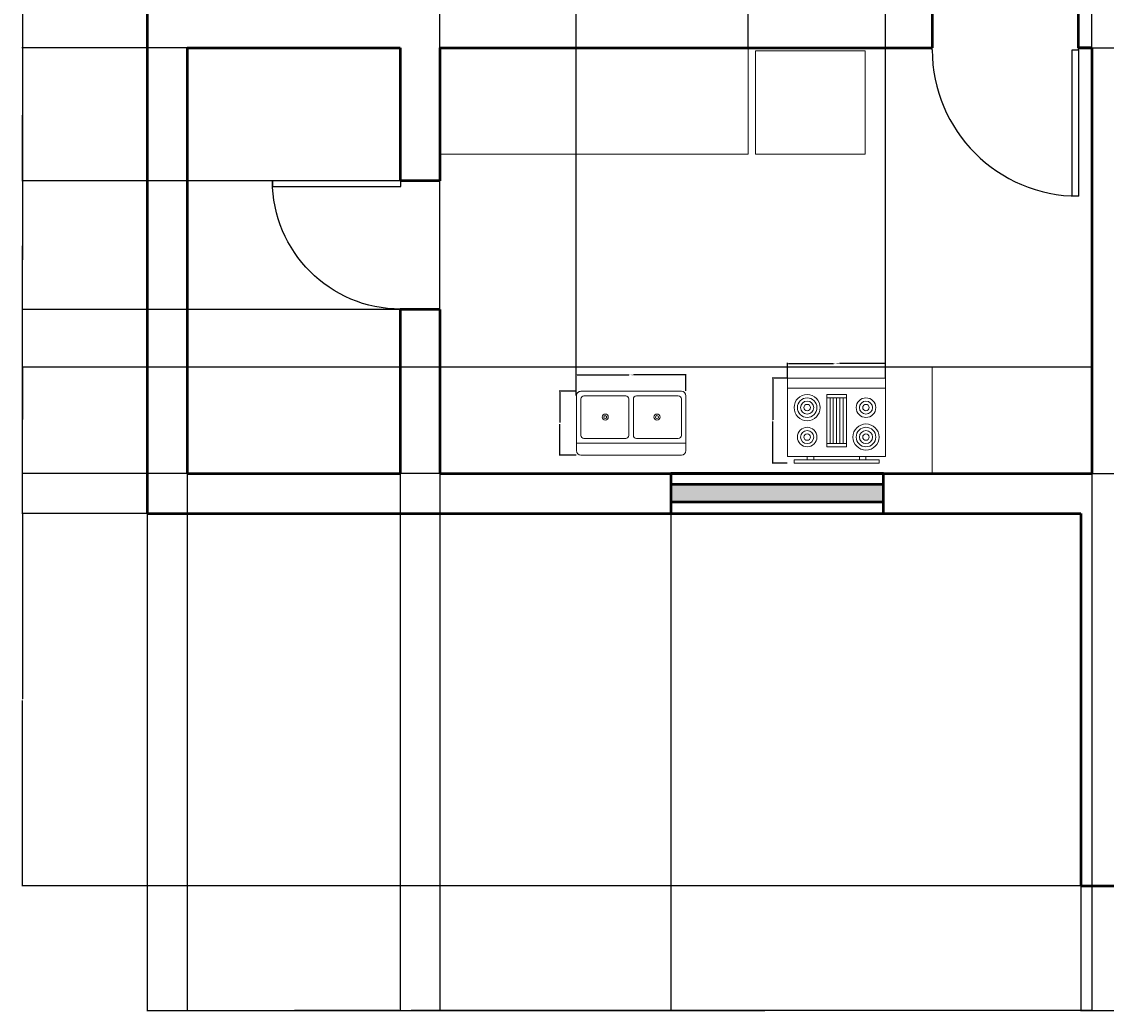
# Model space of a CAD drawing. Units: inches. Extents: x 1974 to 2406, y 1583 to 2170.
# Tile 1 of 6: x 1974 to 2218, y 1583 to 1806. Entities that reach past the tile are written whole.
import ezdxf

# ---------------------------------------------------------------- set-up
doc = ezdxf.new("R2010")
doc.units = ezdxf.units.IN
for name, color, linetype, lineweight in [('A-ANNO-DIMS', 2, 'Continuous', 18), ('A-EQPM', 3, 'Continuous', 18), ('A-FLOR-FIXT', 3, 'Continuous', 18), ('A-GLAZ', 4, 'Continuous', 25), ('door', 60, 'Continuous', 25), ('wall', 240, 'Continuous', 50)]:
    doc.layers.add(name, color=color, linetype=linetype, lineweight=lineweight)
doc.layers.add('A-FLOR-CASE', color=40, linetype='Continuous', lineweight=18, true_color=0xf8d731)
doc.styles.get("Standard").update_dxf_attribs({"font": 'arial.ttf'})
doc.dimstyles.get("Standard").update_dxf_attribs({"dimtxt": 0.18, "dimasz": 0.18, "dimexe": 0.18, "dimexo": 0.0625, "dimgap": 0.09, "dimtad": 0, "dimtih": 1, "dimtoh": 1, "dimdec": 4, "dimzin": 0, "dimdsep": 46, "dimtxsty": 'Standard', "dimcen": 0.09, "dimadec": 0, "dimazin": 0, "dimtfac": 1, "dimtdec": 4, "dimtofl": 0, "dimtmove": 0, "dimatfit": 3, "dimfxl": 1, "dimtolj": 1, "dimtzin": 0, "dimarcsym": 0})

# ---------------------------------------------------------------- blocks, each defined once
blk = doc.blocks.new('*U2')
for p, q in [((0, 0), (0, -6)), ((40, 0), (40, -6))]:
    blk.add_line(p, q)
blk.add_lwpolyline([(0, 0), (0, 40), (1.75, 40), (1.75, 0)], close=True)
blk.add_arc((0, 0), 40, 0, 90)
blk = doc.blocks.new('b')
at = {"layer": 'wall'}
h = blk.add_hatch(color=256, dxfattribs=at)
h.dxf.hatch_style = 1
h.paths.add_polyline_path([(6.5, 0), (2.5, 0), (2.5, -48), (6.5, -48)])
for p, q in [((2.5, 0), (2.5, -48)), ((6.5, 0), (6.5, -48))]:
    blk.add_line(p, q, dxfattribs=at)
blk.add_lwpolyline([(0, -48), (9, -48), (9, 0), (0, 0)], close=True, dxfattribs=at)
blk = doc.blocks.new('Sink-double - 36 in top')
for p, q in [((-18, -4), (18, -4)), ((-0.75, -18.5), (-0.75, -6.5)), ((0.75, -6.5), (0.75, -18.5))]:
    blk.add_line(p, q)
for points in [[(-16.5, 0), (16.5, 0)], [(-18, -19.5), (-18, -1.5)], [(18, -1.5), (18, -19.5)], [(-16.5, -18.5), (-16.5, -6.5)], [(-15.5, -5.5), (-1.75, -5.5)], [(1.75, -5.5), (15.5, -5.5)], [(16.5, -6.5), (16.5, -18.5)], [(16.5, -21), (-16.5, -21)], [(-1.75, -19.5), (-15.5, -19.5)], [(15.5, -19.5), (1.75, -19.5)]]:
    blk.add_lwpolyline(points)
for centre, radius in [((-8.5, -12.5), 1), ((-8.5, -12.5), 0.5), ((8.5, -12.5), 1), ((8.5, -12.5), 0.5)]:
    blk.add_circle(centre, radius)
for centre, radius, start, end in [((-16.5, -1.5), 1.5, 90, 180), ((16.5, -1.5), 1.5, 0, 90), ((-15.5, -6.5), 1, 90, 180), ((-1.75, -6.5), 1, 0, 90), ((1.75, -6.5), 1, 90, 180), ((15.5, -6.5), 1, 0, 90), ((-16.5, -19.5), 1.5, 180, 270), ((-15.5, -18.5), 1, 180, 270), ((-1.75, -18.5), 1, 270, 0), ((1.75, -18.5), 1, 180, 270), ((15.5, -18.5), 1, 270, 0), ((16.5, -19.5), 1.5, 270, 0)]:
    blk.add_arc(centre, radius, start, end)
blk = doc.blocks.new('Range-Oven - 30 in top')
for p, q in [((0, -3), (30, -3)), ((12, -6), (18, -6)), ((13, -20), (13, -6)), ((14, -6), (14, -20)), ((15, -20), (15, -6)), ((16, -6), (16, -20)), ((17, -20), (17, -6)), ((18, -20), (12, -20)), ((6, -24), (6, -25)), ((8, -25), (8, -24)), ((22, -25), (22, -24)), ((24, -24), (24, -25))]:
    blk.add_line(p, q)
for points in [[(0, -24), (0, 0), (30, 0), (30, -24)], [(12, -21), (12, -5), (18, -5), (18, -21)], [(2, -26), (2, -25), (28, -25), (28, -26)]]:
    blk.add_lwpolyline(points, close=True)
for centre, radius in [((6, -9), 4), ((6, -9), 3), ((24, -9), 3), ((6, -9), 2), ((6, -9), 1), ((24, -9), 2), ((24, -9), 1), ((6, -18), 3), ((6, -18), 2), ((24, -18), 4), ((24, -18), 3), ((24, -18), 2), ((6, -18), 1), ((24, -18), 1)]:
    blk.add_circle(centre, radius)
blk = doc.blocks.new('*D38')
at = {"layer": 'A-ANNO-DIMS', "color": 0, "lineweight": -2, "transparency": 16777216}
for p, q in [((2098.9, 1722.59), (2098.9, 1726.41)), ((2099.08, 1726.23), (2110.71, 1726.23)), ((2123.43, 1726.23), (2111.81, 1726.23)), ((2123.61, 1722.59), (2123.61, 1726.41))]:
    blk.add_line(p, q, dxfattribs=at)
at = {"layer": 'A-ANNO-DIMS', "color": 0, "transparency": 16777216}
for points in [[(2099.08, 1726.26), (2099.08, 1726.2), (2098.9, 1726.23)], [(2123.43, 1726.26), (2123.43, 1726.2), (2123.61, 1726.23)]]:
    blk.add_solid(points, dxfattribs=at)
at = {"layer": 'Defpoints', "color": 0, "transparency": 16777216}
for p in [(2098.9, 1726.23), (2098.9, 1722.52), (2123.61, 1722.52)]:
    blk.add_point(p, dxfattribs=at)
at = {"layer": 'A-ANNO-DIMS', "color": 0, "transparency": 16777216, "insert": (2111.26, 1726.23), "char_height": 0.18, "attachment_point": 5}
blk.add_mtext('\\A1;SINK 25', dxfattribs=at)
blk = doc.blocks.new('*D39')
at = {"layer": 'A-ANNO-DIMS', "color": 0, "lineweight": -2, "transparency": 16777216}
for p, q in [((2098.84, 1722.52), (2095.02, 1722.52)), ((2095.2, 1722.34), (2095.2, 1715.5)), ((2095.2, 1708.29), (2095.2, 1715.14)), ((2098.84, 1708.11), (2095.02, 1708.11))]:
    blk.add_line(p, q, dxfattribs=at)
at = {"layer": 'A-ANNO-DIMS', "color": 0, "transparency": 16777216}
for points in [[(2095.17, 1722.34), (2095.23, 1722.34), (2095.2, 1722.52)], [(2095.17, 1708.29), (2095.23, 1708.29), (2095.2, 1708.11)]]:
    blk.add_solid(points, dxfattribs=at)
at = {"layer": 'Defpoints', "color": 0, "transparency": 16777216}
for p in [(2098.9, 1722.52), (2095.2, 1708.11), (2098.9, 1708.11)]:
    blk.add_point(p, dxfattribs=at)
at = {"layer": 'A-ANNO-DIMS', "color": 0, "transparency": 16777216, "insert": (2095.2, 1715.32), "char_height": 0.18, "attachment_point": 5}
blk.add_mtext('\\A1;14', dxfattribs=at)
blk = doc.blocks.new('*D46')
at = {"layer": 'A-ANNO-DIMS', "color": 0, "lineweight": -2, "transparency": 16777216}
for p, q in [((2146.53, 1725.52), (2146.53, 1728.96)), ((2146.71, 1728.78), (2156.89, 1728.78)), ((2168.46, 1728.78), (2158.28, 1728.78)), ((2168.64, 1725.52), (2168.64, 1728.96))]:
    blk.add_line(p, q, dxfattribs=at)
at = {"layer": 'A-ANNO-DIMS', "color": 0, "transparency": 16777216}
for points in [[(2146.71, 1728.81), (2146.71, 1728.75), (2146.53, 1728.78)], [(2168.46, 1728.81), (2168.46, 1728.75), (2168.64, 1728.78)]]:
    blk.add_solid(points, dxfattribs=at)
at = {"layer": 'Defpoints', "color": 0, "transparency": 16777216}
for p in [(2168.64, 1728.78), (2146.53, 1725.46), (2168.64, 1725.46)]:
    blk.add_point(p, dxfattribs=at)
at = {"layer": 'A-ANNO-DIMS', "color": 0, "transparency": 16777216, "insert": (2157.58, 1728.78), "char_height": 0.18, "attachment_point": 5}
blk.add_mtext('\\A1;RANGE 22', dxfattribs=at)
blk = doc.blocks.new('*D47')
at = {"layer": 'A-ANNO-DIMS', "color": 0, "lineweight": -2, "transparency": 16777216}
for p, q in [((2146.47, 1725.46), (2143.03, 1725.46)), ((2143.21, 1725.28), (2143.21, 1716.06)), ((2143.21, 1706.48), (2143.21, 1715.7)), ((2146.47, 1706.3), (2143.03, 1706.3))]:
    blk.add_line(p, q, dxfattribs=at)
at = {"layer": 'A-ANNO-DIMS', "color": 0, "transparency": 16777216}
for points in [[(2143.18, 1725.28), (2143.24, 1725.28), (2143.21, 1725.46)], [(2143.18, 1706.48), (2143.24, 1706.48), (2143.21, 1706.3)]]:
    blk.add_solid(points, dxfattribs=at)
at = {"layer": 'Defpoints', "color": 0, "transparency": 16777216}
for p in [(2143.21, 1725.46), (2146.53, 1725.46), (2146.53, 1706.3)]:
    blk.add_point(p, dxfattribs=at)
at = {"layer": 'A-ANNO-DIMS', "color": 0, "transparency": 16777216, "insert": (2143.21, 1715.88), "char_height": 0.18, "attachment_point": 5}
blk.add_mtext('\\A1;19', dxfattribs=at)
blk = doc.blocks.new('*D57')
at = {"layer": 'A-ANNO-DIMS', "color": 0, "lineweight": -2, "transparency": 16777216}
for p, q in [((2011.1, 1808.99), (1973.86, 1808.99)), ((1974.04, 1808.81), (1974.04, 1752.17)), ((1974.04, 1695.17), (1974.04, 1751.81)), ((2002.1, 1694.99), (1973.86, 1694.99))]:
    blk.add_line(p, q, dxfattribs=at)
at = {"layer": 'A-ANNO-DIMS', "color": 0, "transparency": 16777216}
for points in [[(1974.01, 1808.81), (1974.07, 1808.81), (1974.04, 1808.99)], [(1974.01, 1695.17), (1974.07, 1695.17), (1974.04, 1694.99)]]:
    blk.add_solid(points, dxfattribs=at)
at = {"layer": 'Defpoints', "color": 0, "transparency": 16777216}
for p in [(2011.16, 1808.99), (1974.04, 1694.99), (2002.16, 1694.99)]:
    blk.add_point(p, dxfattribs=at)
at = {"layer": 'A-ANNO-DIMS', "color": 0, "transparency": 16777216, "insert": (1974.04, 1751.99), "char_height": 0.18, "attachment_point": 5}
blk.add_mtext('\\A1;114', dxfattribs=at)
blk = doc.blocks.new('*D58')
at = {"layer": 'A-ANNO-DIMS', "color": 0, "lineweight": -2, "transparency": 16777216}
for p, q in [((2002.1, 1694.99), (1973.86, 1694.99)), ((1974.04, 1694.81), (1974.04, 1653.17)), ((1974.04, 1611.17), (1974.04, 1652.81)), ((2212.6, 1610.99), (1973.86, 1610.99))]:
    blk.add_line(p, q, dxfattribs=at)
at = {"layer": 'A-ANNO-DIMS', "color": 0, "transparency": 16777216}
for points in [[(1974.01, 1694.81), (1974.07, 1694.81), (1974.04, 1694.99)], [(1974.01, 1611.17), (1974.07, 1611.17), (1974.04, 1610.99)]]:
    blk.add_solid(points, dxfattribs=at)
at = {"layer": 'Defpoints', "color": 0, "transparency": 16777216}
for p in [(2002.16, 1694.99), (1974.04, 1610.99), (2212.66, 1610.99)]:
    blk.add_point(p, dxfattribs=at)
at = {"layer": 'A-ANNO-DIMS', "color": 0, "transparency": 16777216, "insert": (1974.04, 1652.99), "char_height": 0.18, "attachment_point": 5}
blk.add_mtext('\\A1;84', dxfattribs=at)
blk = doc.blocks.new('*D61')
at = {"layer": 'A-ANNO-DIMS', "color": 0, "lineweight": -2, "transparency": 16777216}
for p, q in [((2002.16, 1694.93), (2002.16, 1582.69)), ((2212.66, 1610.93), (2212.66, 1582.69)), ((2002.34, 1582.87), (2107.01, 1582.87)), ((2212.48, 1582.87), (2107.8, 1582.87))]:
    blk.add_line(p, q, dxfattribs=at)
at = {"layer": 'A-ANNO-DIMS', "color": 0, "transparency": 16777216}
for points in [[(2002.34, 1582.9), (2002.34, 1582.84), (2002.16, 1582.87)], [(2212.48, 1582.9), (2212.48, 1582.84), (2212.66, 1582.87)]]:
    blk.add_solid(points, dxfattribs=at)
at = {"layer": 'Defpoints', "color": 0, "transparency": 16777216}
for p in [(2002.16, 1694.99), (2212.66, 1610.99), (2212.66, 1582.87)]:
    blk.add_point(p, dxfattribs=at)
at = {"layer": 'A-ANNO-DIMS', "color": 0, "transparency": 16777216, "insert": (2107.41, 1582.87), "char_height": 0.18, "attachment_point": 5}
blk.add_mtext('\\A1;210.5', dxfattribs=at)
blk = doc.blocks.new('*D62')
at = {"layer": 'A-ANNO-DIMS', "color": 0, "lineweight": -2, "transparency": 16777216}
for p, q in [((2212.66, 1610.93), (2212.66, 1582.69)), ((2377.66, 1610.93), (2377.66, 1582.69)), ((2212.84, 1582.87), (2294.88, 1582.87)), ((2377.48, 1582.87), (2295.44, 1582.87))]:
    blk.add_line(p, q, dxfattribs=at)
at = {"layer": 'A-ANNO-DIMS', "color": 0, "transparency": 16777216}
for points in [[(2212.84, 1582.9), (2212.84, 1582.84), (2212.66, 1582.87)], [(2377.48, 1582.9), (2377.48, 1582.84), (2377.66, 1582.87)]]:
    blk.add_solid(points, dxfattribs=at)
at = {"layer": 'Defpoints', "color": 0, "transparency": 16777216}
for p in [(2212.66, 1610.99), (2377.66, 1610.99), (2377.66, 1582.87)]:
    blk.add_point(p, dxfattribs=at)
at = {"layer": 'A-ANNO-DIMS', "color": 0, "transparency": 16777216, "insert": (2295.16, 1582.87), "char_height": 0.18, "attachment_point": 5}
blk.add_mtext('\\A1;165', dxfattribs=at)
blk = doc.blocks.new('*D83')
at = {"layer": 'A-ANNO-DIMS', "color": 0, "lineweight": -2, "transparency": 16777216}
for p, q in [((2011.16, 1703.93), (2011.16, 1582.69)), ((2059.16, 1703.93), (2059.16, 1582.69)), ((2011.34, 1582.87), (2034.94, 1582.87)), ((2058.98, 1582.87), (2035.38, 1582.87))]:
    blk.add_line(p, q, dxfattribs=at)
at = {"layer": 'A-ANNO-DIMS', "color": 0, "transparency": 16777216}
for points in [[(2011.34, 1582.9), (2011.34, 1582.84), (2011.16, 1582.87)], [(2058.98, 1582.9), (2058.98, 1582.84), (2059.16, 1582.87)]]:
    blk.add_solid(points, dxfattribs=at)
at = {"layer": 'Defpoints', "color": 0, "transparency": 16777216}
for p in [(2011.16, 1703.99), (2059.16, 1703.99), (2059.16, 1582.87)]:
    blk.add_point(p, dxfattribs=at)
at = {"layer": 'A-ANNO-DIMS', "color": 0, "transparency": 16777216, "insert": (2035.16, 1582.87), "char_height": 0.18, "attachment_point": 5}
blk.add_mtext('\\A1;48', dxfattribs=at)
blk = doc.blocks.new('*D84')
at = {"layer": 'A-ANNO-DIMS', "color": 0, "lineweight": -2, "transparency": 16777216}
for p, q in [((2059.16, 1703.93), (2059.16, 1582.69)), ((2068.16, 1703.93), (2068.16, 1582.69)), ((2059.34, 1582.87), (2063.51, 1582.87)), ((2067.98, 1582.87), (2063.81, 1582.87))]:
    blk.add_line(p, q, dxfattribs=at)
at = {"layer": 'A-ANNO-DIMS', "color": 0, "transparency": 16777216}
for points in [[(2059.34, 1582.9), (2059.34, 1582.84), (2059.16, 1582.87)], [(2067.98, 1582.9), (2067.98, 1582.84), (2068.16, 1582.87)]]:
    blk.add_solid(points, dxfattribs=at)
at = {"layer": 'Defpoints', "color": 0, "transparency": 16777216}
for p in [(2059.16, 1703.99), (2068.16, 1703.99), (2068.16, 1582.87)]:
    blk.add_point(p, dxfattribs=at)
at = {"layer": 'A-ANNO-DIMS', "color": 0, "transparency": 16777216, "insert": (2063.66, 1582.87), "char_height": 0.18, "attachment_point": 5}
blk.add_mtext('\\A1;9', dxfattribs=at)
blk = doc.blocks.new('*D85')
at = {"layer": 'A-ANNO-DIMS', "color": 0, "lineweight": -2, "transparency": 16777216}
for p, q in [((2068.16, 1703.93), (2068.16, 1582.69)), ((2215.16, 1703.93), (2215.16, 1582.69)), ((2068.34, 1582.87), (2141.38, 1582.87)), ((2214.98, 1582.87), (2141.94, 1582.87))]:
    blk.add_line(p, q, dxfattribs=at)
at = {"layer": 'A-ANNO-DIMS', "color": 0, "transparency": 16777216}
for points in [[(2068.34, 1582.9), (2068.34, 1582.84), (2068.16, 1582.87)], [(2214.98, 1582.9), (2214.98, 1582.84), (2215.16, 1582.87)]]:
    blk.add_solid(points, dxfattribs=at)
at = {"layer": 'Defpoints', "color": 0, "transparency": 16777216}
for p in [(2068.16, 1703.99), (2215.16, 1703.99), (2215.16, 1582.87)]:
    blk.add_point(p, dxfattribs=at)
at = {"layer": 'A-ANNO-DIMS', "color": 0, "transparency": 16777216, "insert": (2141.66, 1582.87), "char_height": 0.18, "attachment_point": 5}
blk.add_mtext('\\A1;147', dxfattribs=at)
blk = doc.blocks.new('*D86')
at = {"layer": 'A-ANNO-DIMS', "color": 0, "lineweight": -2, "transparency": 16777216}
for p, q in [((2215.22, 1799.99), (2405.96, 1799.99)), ((2405.78, 1799.81), (2405.78, 1752.17)), ((2405.78, 1704.17), (2405.78, 1751.81)), ((2215.22, 1703.99), (2405.96, 1703.99))]:
    blk.add_line(p, q, dxfattribs=at)
at = {"layer": 'A-ANNO-DIMS', "color": 0, "transparency": 16777216}
for points in [[(2405.75, 1799.81), (2405.81, 1799.81), (2405.78, 1799.99)], [(2405.75, 1704.17), (2405.81, 1704.17), (2405.78, 1703.99)]]:
    blk.add_solid(points, dxfattribs=at)
at = {"layer": 'Defpoints', "color": 0, "transparency": 16777216}
for p in [(2215.16, 1799.99), (2215.16, 1703.99), (2405.78, 1703.99)]:
    blk.add_point(p, dxfattribs=at)
at = {"layer": 'A-ANNO-DIMS', "color": 0, "transparency": 16777216, "insert": (2405.78, 1751.99), "char_height": 0.18, "attachment_point": 5}
blk.add_mtext('\\A1;96', dxfattribs=at)
blk = doc.blocks.new('*D87')
at = {"layer": 'A-ANNO-DIMS', "color": 0, "lineweight": -2, "transparency": 16777216}
for p, q in [((2011.1, 1799.99), (1973.86, 1799.99)), ((1974.04, 1799.81), (1974.04, 1785.17)), ((1974.04, 1770.17), (1974.04, 1784.81)), ((2059.1, 1769.99), (1973.86, 1769.99))]:
    blk.add_line(p, q, dxfattribs=at)
at = {"layer": 'A-ANNO-DIMS', "color": 0, "transparency": 16777216}
for points in [[(1974.01, 1799.81), (1974.07, 1799.81), (1974.04, 1799.99)], [(1974.01, 1770.17), (1974.07, 1770.17), (1974.04, 1769.99)]]:
    blk.add_solid(points, dxfattribs=at)
at = {"layer": 'Defpoints', "color": 0, "transparency": 16777216}
for p in [(2011.16, 1799.99), (1974.04, 1769.99), (2059.16, 1769.99)]:
    blk.add_point(p, dxfattribs=at)
at = {"layer": 'A-ANNO-DIMS', "color": 0, "transparency": 16777216, "insert": (1974.04, 1784.99), "char_height": 0.18, "attachment_point": 5}
blk.add_mtext('\\A1;30', dxfattribs=at)
blk = doc.blocks.new('*D88')
at = {"layer": 'A-ANNO-DIMS', "color": 0, "lineweight": -2, "transparency": 16777216}
for p, q in [((2059.1, 1769.99), (1973.86, 1769.99)), ((1974.04, 1769.81), (1974.04, 1755.67)), ((1974.04, 1741.17), (1974.04, 1755.31)), ((2059.1, 1740.99), (1973.86, 1740.99))]:
    blk.add_line(p, q, dxfattribs=at)
at = {"layer": 'A-ANNO-DIMS', "color": 0, "transparency": 16777216}
for points in [[(1974.01, 1769.81), (1974.07, 1769.81), (1974.04, 1769.99)], [(1974.01, 1741.17), (1974.07, 1741.17), (1974.04, 1740.99)]]:
    blk.add_solid(points, dxfattribs=at)
at = {"layer": 'Defpoints', "color": 0, "transparency": 16777216}
for p in [(2059.16, 1769.99), (1974.04, 1740.99), (2059.16, 1740.99)]:
    blk.add_point(p, dxfattribs=at)
at = {"layer": 'A-ANNO-DIMS', "color": 0, "transparency": 16777216, "insert": (1974.04, 1755.49), "char_height": 0.18, "attachment_point": 5}
blk.add_mtext('\\A1;29', dxfattribs=at)
blk = doc.blocks.new('*D90')
at = {"layer": 'A-ANNO-DIMS', "color": 0, "lineweight": -2, "transparency": 16777216}
for p, q in [((2215.1, 1727.99), (1973.86, 1727.99)), ((1974.04, 1727.81), (1974.04, 1716.17)), ((1974.04, 1704.17), (1974.04, 1715.81)), ((2215.1, 1703.99), (1973.86, 1703.99))]:
    blk.add_line(p, q, dxfattribs=at)
at = {"layer": 'A-ANNO-DIMS', "color": 0, "transparency": 16777216}
for points in [[(1974.01, 1727.81), (1974.07, 1727.81), (1974.04, 1727.99)], [(1974.01, 1704.17), (1974.07, 1704.17), (1974.04, 1703.99)]]:
    blk.add_solid(points, dxfattribs=at)
at = {"layer": 'Defpoints', "color": 0, "transparency": 16777216}
for p in [(1974.04, 1727.99), (2215.16, 1727.99), (2215.16, 1703.99)]:
    blk.add_point(p, dxfattribs=at)
at = {"layer": 'A-ANNO-DIMS', "color": 0, "transparency": 16777216, "insert": (1974.04, 1715.99), "char_height": 0.18, "attachment_point": 5}
blk.add_mtext('\\A1;24', dxfattribs=at)
blk = doc.blocks.new('*D91')
at = {"layer": 'A-ANNO-DIMS', "color": 0, "lineweight": -2, "transparency": 16777216}
for p, q in [((2002.16, 1694.93), (2002.16, 1582.69)), ((2120.19, 1694.93), (2120.19, 1582.69)), ((2002.34, 1582.87), (2060.72, 1582.87)), ((2120.01, 1582.87), (2061.63, 1582.87))]:
    blk.add_line(p, q, dxfattribs=at)
at = {"layer": 'A-ANNO-DIMS', "color": 0, "transparency": 16777216}
for points in [[(2002.34, 1582.9), (2002.34, 1582.84), (2002.16, 1582.87)], [(2120.01, 1582.9), (2120.01, 1582.84), (2120.19, 1582.87)]]:
    blk.add_solid(points, dxfattribs=at)
at = {"layer": 'Defpoints', "color": 0, "transparency": 16777216}
for p in [(2002.16, 1694.99), (2120.19, 1694.99), (2120.19, 1582.87)]:
    blk.add_point(p, dxfattribs=at)
at = {"layer": 'A-ANNO-DIMS', "color": 0, "transparency": 16777216, "insert": (2061.17, 1582.87), "char_height": 0.18, "attachment_point": 5}
blk.add_mtext('\\A1;118.03', dxfattribs=at)
blk = doc.blocks.new('*D92')
at = {"layer": 'A-ANNO-DIMS', "color": 0, "lineweight": -2, "transparency": 16777216}
for p, q in [((2168.64, 1725.52), (2168.64, 2170.29)), ((2168.82, 2170.11), (2191.5, 2170.11)), ((2214.98, 2170.11), (2192.3, 2170.11)), ((2215.16, 1728.05), (2215.16, 2170.29))]:
    blk.add_line(p, q, dxfattribs=at)
at = {"layer": 'A-ANNO-DIMS', "color": 0, "transparency": 16777216}
for points in [[(2168.82, 2170.14), (2168.82, 2170.08), (2168.64, 2170.11)], [(2214.98, 2170.14), (2214.98, 2170.08), (2215.16, 2170.11)]]:
    blk.add_solid(points, dxfattribs=at)
at = {"layer": 'Defpoints', "color": 0, "transparency": 16777216}
for p in [(2215.16, 2170.11), (2215.16, 1727.99), (2168.64, 1725.46)]:
    blk.add_point(p, dxfattribs=at)
at = {"layer": 'A-ANNO-DIMS', "color": 0, "transparency": 16777216, "insert": (2191.9, 2170.11), "char_height": 0.18, "attachment_point": 5}
blk.add_mtext('\\A1;46.52', dxfattribs=at)
blk = doc.blocks.new('*D93')
at = {"layer": 'A-ANNO-DIMS', "color": 0, "lineweight": -2, "transparency": 16777216}
for p, q in [((2068.16, 1728.05), (2068.16, 2170.29)), ((2068.34, 2170.11), (2083.07, 2170.11)), ((2098.72, 2170.11), (2083.99, 2170.11)), ((2098.9, 1721.56), (2098.9, 2170.29))]:
    blk.add_line(p, q, dxfattribs=at)
at = {"layer": 'A-ANNO-DIMS', "color": 0, "transparency": 16777216}
for points in [[(2068.34, 2170.14), (2068.34, 2170.08), (2068.16, 2170.11)], [(2098.72, 2170.14), (2098.72, 2170.08), (2098.9, 2170.11)]]:
    blk.add_solid(points, dxfattribs=at)
at = {"layer": 'Defpoints', "color": 0, "transparency": 16777216}
for p in [(2098.9, 2170.11), (2068.16, 1727.99), (2098.9, 1721.49)]:
    blk.add_point(p, dxfattribs=at)
at = {"layer": 'A-ANNO-DIMS', "color": 0, "transparency": 16777216, "insert": (2083.53, 2170.11), "char_height": 0.18, "attachment_point": 5}
blk.add_mtext('\\A1;30.746', dxfattribs=at)
blk = doc.blocks.new('*D94')
at = {"layer": 'A-ANNO-DIMS', "color": 0, "lineweight": -2, "transparency": 16777216}
for p, q in [((2068.16, 1800.05), (2068.16, 2170.29)), ((2068.34, 2170.11), (2102.58, 2170.11)), ((2137.48, 2170.11), (2103.23, 2170.11)), ((2137.66, 1800.05), (2137.66, 2170.29))]:
    blk.add_line(p, q, dxfattribs=at)
at = {"layer": 'A-ANNO-DIMS', "color": 0, "transparency": 16777216}
for points in [[(2068.34, 2170.14), (2068.34, 2170.08), (2068.16, 2170.11)], [(2137.48, 2170.14), (2137.48, 2170.08), (2137.66, 2170.11)]]:
    blk.add_solid(points, dxfattribs=at)
at = {"layer": 'Defpoints', "color": 0, "transparency": 16777216}
for p in [(2137.66, 2170.11), (2068.16, 1799.99), (2137.66, 1799.99)]:
    blk.add_point(p, dxfattribs=at)
at = {"layer": 'A-ANNO-DIMS', "color": 0, "transparency": 16777216, "insert": (2102.91, 2170.11), "char_height": 0.18, "attachment_point": 5}
blk.add_mtext('\\A1;69.5', dxfattribs=at)

msp = doc.modelspace()

# ---------------------------------------------------------------- linework, layer by layer
at = {"layer": 'A-EQPM'}
msp.add_lwpolyline([(2139.3345, 1799.2965), (2164.0041, 1799.2965), (2164.0041, 1775.9951), (2139.3345, 1775.9951)], close=True, dxfattribs=at)
at = {"layer": 'A-FLOR-CASE'}
for p, q in [((2068.1581, 1799.9921), (2068.1581, 1775.9921)), ((2137.6581, 1775.9921), (2137.6581, 1799.9921)), ((2068.1581, 1775.9921), (2137.6581, 1775.9921)), ((2179.149, 1727.9921), (2068.1581, 1727.9921)), ((2215.1581, 1727.9921), (2179.149, 1727.9921)), ((2179.149, 1727.9921), (2179.149, 1703.9921)), ((2215.1581, 1703.9921), (2215.1581, 1727.9921))]:
    msp.add_line(p, q, dxfattribs=at)
for points in [[(2068.1581, 1799.9921), (2137.6581, 1799.9921), (2137.6581, 1775.9921), (2068.1581, 1775.9921)], [(2068.1581, 1703.9921), (2179.149, 1703.9921), (2179.149, 1727.9921), (2068.1581, 1727.9921)], [(2215.1581, 1703.9921), (2179.149, 1703.9921), (2179.149, 1727.9921), (2215.1581, 1727.9921)]]:
    msp.add_lwpolyline(points, close=True, dxfattribs=at)
at = {"layer": 'wall'}
for p, q in [((2002.1581, 2141.9921), (2002.1581, 1694.9921)), ((2179.1581, 1808.9921), (2179.1581, 1799.9921)), ((2212.1581, 1799.9921), (2212.1581, 1808.9921)), ((2011.1581, 1799.9921), (2059.1581, 1799.9921)), ((2011.1581, 1799.9921), (2011.1581, 1703.9921)), ((2059.1581, 1799.9921), (2059.1581, 1769.9921)), ((2068.1581, 1799.9921), (2068.1581, 1769.9921)), ((2068.1581, 1799.9921), (2137.6581, 1799.9921)), ((2137.6581, 1799.9921), (2179.1581, 1799.9921)), ((2215.1581, 1799.9921), (2212.1581, 1799.9921)), ((2212.1581, 1799.9921), (2215.1581, 1799.9921)), ((2215.1581, 1799.9921), (2215.1581, 1703.9921)), ((2068.1581, 1775.9921), (2068.1581, 1769.9921)), ((2068.1581, 1769.9921), (2059.1581, 1769.9921)), ((2068.1581, 1740.9921), (2059.1581, 1740.9921)), ((2059.1581, 1740.9921), (2059.1581, 1703.9921)), ((2068.1581, 1740.9921), (2068.1581, 1703.9921)), ((2011.1581, 1703.9921), (2059.1581, 1703.9921)), ((2068.1581, 1703.9921), (2215.1581, 1703.9921)), ((2002.1581, 1694.9921), (2212.6581, 1694.9921)), ((2212.6581, 1694.9921), (2212.6581, 1610.9921)), ((2212.6581, 1610.9921), (2377.6581, 1610.9921))]:
    msp.add_line(p, q, dxfattribs=at)

# ---------------------------------------------------------------- block references
at = {"layer": 'A-EQPM', "xscale": 0.736975325430527, "yscale": 0.736975325430527, "zscale": 0.736975325430527}
msp.add_blockref('Range-Oven - 30 in top', (2146.5301, 1725.4624), dxfattribs=at)
at = {"layer": 'A-FLOR-FIXT', "xscale": 0.6863619148228619, "yscale": 0.6863619148228619, "zscale": 0.6863619148228619, "rotation": 180}
msp.add_blockref('Sink-double - 36 in top', (2111.2584, 1708.1103), dxfattribs=at)
at = {"layer": 'A-GLAZ', "rotation": 270}
msp.add_blockref('b', (2168.1886, 1703.9921), dxfattribs=at)
at = {"layer": 'door'}
for p, xscale, yscale, zscale, rotation in [((2212.1581, 1799.5407), 0.8252274917434117, 0.8252274917434117, 0.8252274917434117, 179.9999999999992), ((2059.3166, 1769.9921), -0.7235736985599088, 0.7235736985599088, 0.7235736985599088, 90)]:
    msp.add_blockref('*U2', p, dxfattribs=dict(at, xscale=xscale, yscale=yscale, zscale=zscale, rotation=rotation))

# ---------------------------------------------------------------- dimensions: what is measured, and where the dimension line sits
at = {"layer": 'A-ANNO-DIMS'}
for base, p1, p2, override, picture, middle in [((2098.9039, 2170.1096), (2068.1581, 1727.9921), (2098.9039, 1721.4943), {"dimdec": 3, "dimlfac": 1, "dimrnd": 0, "dimzin": 0, "dimdsep": 46, "dimlunit": 2}, '*D93', (2083.531, 2170.1096)), ((2137.6581, 2170.1096), (2068.1581, 1799.9921), (2137.6581, 1799.9921), {"dimdec": 1, "dimlfac": 1, "dimrnd": 0, "dimzin": 0, "dimdsep": 46, "dimlunit": 2}, '*D94', (2102.9081, 2170.1096)), ((2215.1581, 2170.1096), (2168.6394, 1725.4624), (2215.1581, 1727.9921), {"dimdec": 2, "dimlfac": 1, "dimrnd": 0, "dimzin": 0, "dimdsep": 46, "dimlunit": 2}, '*D92', (2191.8987, 2170.1096)), ((2059.1581, 1582.8746), (2011.1581, 1703.9921), (2059.1581, 1703.9921), {"dimdec": 0, "dimlfac": 1, "dimrnd": 0, "dimzin": 0, "dimdsep": 46, "dimlunit": 2}, '*D83', (2035.1581, 1582.8746)), ((2068.1581, 1582.8746), (2059.1581, 1703.9921), (2068.1581, 1703.9921), {"dimdec": 0, "dimlfac": 1, "dimrnd": 0, "dimzin": 0, "dimdsep": 46, "dimlunit": 2}, '*D84', (2063.6581, 1582.8746)), ((2215.1581, 1582.8746), (2068.1581, 1703.9921), (2215.1581, 1703.9921), {"dimdec": 0, "dimlfac": 1, "dimrnd": 0, "dimzin": 0, "dimdsep": 46, "dimlunit": 2}, '*D85', (2141.6581, 1582.8746)), ((2212.6581, 1582.8746), (2002.1581, 1694.9921), (2212.6581, 1610.9921), {"dimdec": 1, "dimlfac": 1, "dimrnd": 0, "dimzin": 0, "dimdsep": 46, "dimlunit": 2}, '*D61', (2107.4081, 1582.8746)), ((2120.1886, 1582.8746), (2002.1581, 1694.9921), (2120.1886, 1694.9921), {"dimdec": 2, "dimlfac": 1, "dimrnd": 0, "dimzin": 0, "dimdsep": 46, "dimlunit": 2}, '*D91', (2061.1733, 1582.8746)), ((2377.6581, 1582.8746), (2212.6581, 1610.9921), (2377.6581, 1610.9921), {"dimdec": 0, "dimlfac": 1, "dimrnd": 0, "dimzin": 0, "dimdsep": 46, "dimlunit": 2}, '*D62', (2295.1581, 1582.8746))]:
    dim = msp.add_linear_dim(base=base, p1=p1, p2=p2, dimstyle='Standard', override=override, dxfattribs=at)
    dim.commit()
    dim.dimension.update_dxf_attribs({"geometry": picture, "text_midpoint": middle})
for base, p1, p2, angle, picture, middle in [((1974.0406, 1694.9921), (2011.1581, 1808.9921), (2002.1581, 1694.9921), 90, '*D57', (1974.0406, 1751.9921)), ((1974.0406, 1769.9921), (2011.1581, 1799.9921), (2059.1581, 1769.9921), 90, '*D87', (1974.0406, 1784.9921)), ((2405.7756, 1703.9921), (2215.1581, 1799.9921), (2215.1581, 1703.9921), 90, '*D86', (2405.7756, 1751.9921)), ((1974.0406, 1740.9921), (2059.1581, 1769.9921), (2059.1581, 1740.9921), 90, '*D88', (1974.0406, 1755.4921)), ((1974.0406, 1727.9921), (2215.1581, 1703.9921), (2215.1581, 1727.9921), 90, '*D90', (1974.0406, 1715.9921)), ((2143.2137, 1725.4624), (2146.5301, 1706.301), (2146.5301, 1725.4624), 90, '*D47', (2143.2137, 1715.8817)), ((2095.1976, 1708.1103), (2098.9039, 1722.5239), (2098.9039, 1708.1103), 270, '*D39', (2095.1976, 1715.3171)), ((1974.0406, 1610.9921), (2002.1581, 1694.9921), (2212.6581, 1610.9921), 90, '*D58', (1974.0406, 1652.9921))]:
    dim = msp.add_linear_dim(base=base, p1=p1, p2=p2, angle=angle, dimstyle='Standard', override={"dimdec": 0, "dimlfac": 1, "dimrnd": 0, "dimzin": 0, "dimdsep": 46, "dimlunit": 2}, dxfattribs=at)
    dim.commit()
    dim.dimension.update_dxf_attribs({"geometry": picture, "text_midpoint": middle})
dim = msp.add_linear_dim(base=(2168.6394, 1728.7788), p1=(2146.5301, 1725.4624), p2=(2168.6394, 1725.4624), text='RANGE <>', dimstyle='Standard', override={"dimdec": 0, "dimlfac": 1, "dimrnd": 0, "dimzin": 0, "dimdsep": 46, "dimlunit": 2}, dxfattribs=at)
dim.commit()
dim.dimension.update_dxf_attribs({"geometry": '*D46', "text_midpoint": (2157.5848, 1728.7788)})
dim = msp.add_linear_dim(base=(2098.9039, 1726.2302), p1=(2123.613, 1722.5239), p2=(2098.9039, 1722.5239), angle=180, text='SINK <>', dimstyle='Standard', override={"dimdec": 0, "dimlfac": 1, "dimrnd": 0, "dimzin": 0, "dimdsep": 46, "dimlunit": 2}, dxfattribs=at)
dim.commit()
dim.dimension.update_dxf_attribs({"geometry": '*D38', "text_midpoint": (2111.2584, 1726.2302)})

doc.saveas('drawing.dxf')
